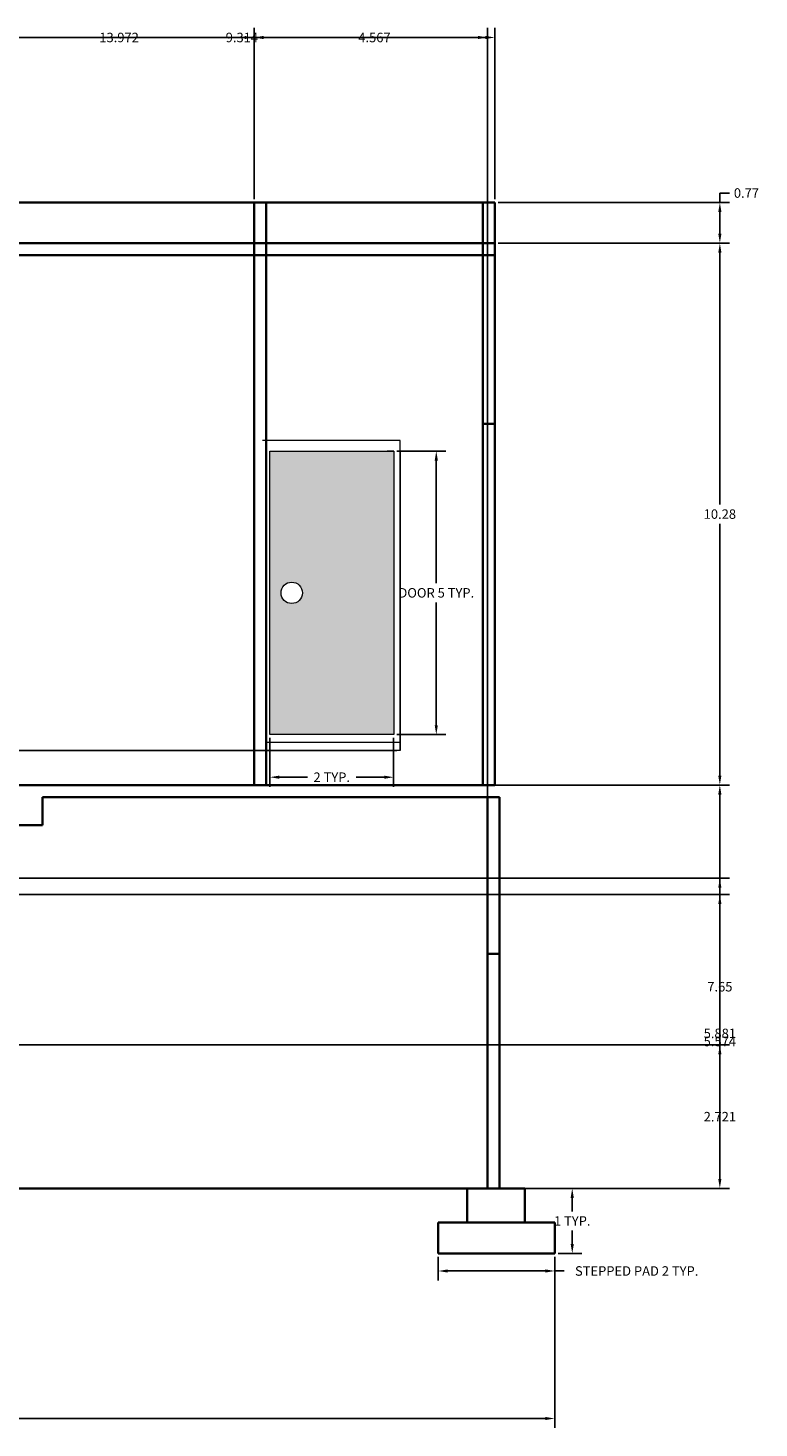
# Model space of a CAD drawing. Units: metres. Extents: x 1976.6 to 2045, y 823.7 to 850.3.
# Tile 3 of 3: x 2031.2 to 2045, y 823.7 to 850.3. Entities that reach past the tile are written whole.
import ezdxf

# ---------------------------------------------------------------- set-up
doc = ezdxf.new("R2010")
doc.units = ezdxf.units.M
for name, color, linetype, lineweight in [('A-ANNO-DIMS', 2, 'Continuous', 18), ('A-DOOR', 3, 'Continuous', 18), ('A-FLOR', 7, 'Continuous', 35), ('A-ROOF', 7, 'Continuous', 35), ('A-WALL', 7, 'Continuous', 35), ('A-WALL-PRPT', 7, 'Continuous', 35), ('S-BEAM', 1, 'Continuous', 35), ('S-FNDN', 1, 'Continuous', 35)]:
    doc.layers.add(name, color=color, linetype=linetype, lineweight=lineweight)
doc.styles.get("Standard").update_dxf_attribs({"font": 'arial.ttf'})
doc.dimstyles.get("Standard").update_dxf_attribs({"dimtxt": 0.18, "dimasz": 0.18, "dimexe": 0.18, "dimexo": 0.0625, "dimgap": 0.09, "dimtad": 0, "dimtih": 1, "dimtoh": 1, "dimdec": 4, "dimzin": 0, "dimdsep": 46, "dimtxsty": 'Standard', "dimcen": 0.09, "dimadec": 0, "dimazin": 0, "dimtfac": 1, "dimtdec": 4, "dimtofl": 0, "dimtmove": 0, "dimatfit": 3, "dimfxl": 1, "dimtolj": 1, "dimtzin": 0, "dimarcsym": 0})

# ---------------------------------------------------------------- blocks, each defined once
blk = doc.blocks.new('FNDN-STEPPED-PAD')
for p, q in [((0.547, 1.235), (0.547, 0.59)), ((1.641, 0.59), (1.641, 1.235)), ((0.547, 0.59), (0, 0.59)), ((0, 0.59), (0, 0)), ((0.547, 0.59), (1.641, 0.59)), ((2.209, 0.59), (1.641, 0.59)), ((2.209, 0), (2.209, 0.59)), ((0, 0), (2.209, 0))]:
    blk.add_line(p, q)
blk = doc.blocks.new('DOOR-SINGLE-LEAF')
h = blk.add_hatch(color=256)
h.dxf.hatch_style = 1
h.paths.add_polyline_path([(2.349, 5.38), (2.224, 5.38), (0, 5.38), (0, 0), (2.349, 0)])
h.paths.add_polyline_path([(0.213, 2.69, -1), (0.619, 2.69, -1)], flags=16)
for p, q in [((2.349, 5.38), (2.224, 5.38)), ((2.224, 5.38), (2.349, 5.38)), ((2.349, 5.38), (2.349, 0)), ((2.349, 0), (0, 0))]:
    blk.add_line(p, q)
blk.add_lwpolyline([(0, 0), (0, 5.38), (2.349, 5.38)])
blk.add_circle((0.416, 2.69), 0.203)
blk = doc.blocks.new('*D6')
at = {"layer": 'A-ANNO-DIMS', "color": 0, "lineweight": -2, "transparency": 16777216}
for p, q in [((2038.945, 826.987), (2038.945, 826.538)), ((2041.154, 826.987), (2041.154, 826.538)), ((2039.125, 826.718), (2040.974, 826.718)), ((2041.154, 826.718), (2041.334, 826.718))]:
    blk.add_line(p, q, dxfattribs=at)
at = {"layer": 'A-ANNO-DIMS', "color": 0, "transparency": 16777216}
for points in [[(2039.125, 826.748), (2039.125, 826.688), (2038.945, 826.718)], [(2040.974, 826.748), (2040.974, 826.688), (2041.154, 826.718)]]:
    blk.add_solid(points, dxfattribs=at)
at = {"layer": 'Defpoints', "color": 0, "transparency": 16777216}
for p in [(2038.945, 827.05), (2041.154, 827.05), (2041.154, 826.718)]:
    blk.add_point(p, dxfattribs=at)
at = {"layer": 'A-ANNO-DIMS', "color": 0, "transparency": 16777216, "insert": (2042.707, 826.718), "char_height": 0.18, "attachment_point": 5}
blk.add_mtext('\\A1;STEPPED PAD 2 TYP.', dxfattribs=at)
blk = doc.blocks.new('*D7')
at = {"layer": 'A-ANNO-DIMS', "color": 0, "lineweight": -2, "transparency": 16777216}
for p, q in [((2041.216, 828.285), (2041.665, 828.285)), ((2041.485, 828.105), (2041.485, 827.848)), ((2041.485, 827.23), (2041.485, 827.487)), ((2041.216, 827.05), (2041.665, 827.05))]:
    blk.add_line(p, q, dxfattribs=at)
at = {"layer": 'A-ANNO-DIMS', "color": 0, "transparency": 16777216}
for points in [[(2041.455, 828.105), (2041.515, 828.105), (2041.485, 828.285)], [(2041.455, 827.23), (2041.515, 827.23), (2041.485, 827.05)]]:
    blk.add_solid(points, dxfattribs=at)
at = {"layer": 'Defpoints', "color": 0, "transparency": 16777216}
for p in [(2041.154, 828.285), (2041.485, 828.285), (2041.154, 827.05)]:
    blk.add_point(p, dxfattribs=at)
at = {"layer": 'A-ANNO-DIMS', "color": 0, "transparency": 16777216, "insert": (2041.485, 827.667), "char_height": 0.18, "attachment_point": 5}
blk.add_mtext('\\A1;1 TYP.', dxfattribs=at)
blk = doc.blocks.new('*D12')
at = {"layer": 'A-ANNO-DIMS', "color": 0, "lineweight": -2, "transparency": 16777216}
for p, q in [((2038.162, 842.271), (2039.087, 842.271)), ((2038.907, 842.091), (2038.907, 839.764)), ((2038.907, 837.071), (2038.907, 839.398)), ((2038.162, 836.891), (2039.087, 836.891))]:
    blk.add_line(p, q, dxfattribs=at)
at = {"layer": 'A-ANNO-DIMS', "color": 0, "transparency": 16777216}
for points in [[(2038.877, 842.091), (2038.937, 842.091), (2038.907, 842.271)], [(2038.877, 837.071), (2038.937, 837.071), (2038.907, 836.891)]]:
    blk.add_solid(points, dxfattribs=at)
at = {"layer": 'Defpoints', "color": 0, "transparency": 16777216}
for p in [(2038.099, 842.271), (2038.907, 842.271), (2038.099, 836.891)]:
    blk.add_point(p, dxfattribs=at)
at = {"layer": 'A-ANNO-DIMS', "color": 0, "transparency": 16777216, "insert": (2038.907, 839.581), "char_height": 0.18, "attachment_point": 5}
blk.add_mtext('\\A1;DOOR 5 TYP.', dxfattribs=at)
blk = doc.blocks.new('*D13')
at = {"layer": 'A-ANNO-DIMS', "color": 0, "lineweight": -2, "transparency": 16777216}
for p, q in [((2035.75, 836.828), (2035.75, 835.904)), ((2038.099, 836.828), (2038.099, 835.904)), ((2035.93, 836.084), (2036.465, 836.084)), ((2037.919, 836.084), (2037.385, 836.084))]:
    blk.add_line(p, q, dxfattribs=at)
at = {"layer": 'A-ANNO-DIMS', "color": 0, "transparency": 16777216}
for points in [[(2035.93, 836.114), (2035.93, 836.054), (2035.75, 836.084)], [(2037.919, 836.114), (2037.919, 836.054), (2038.099, 836.084)]]:
    blk.add_solid(points, dxfattribs=at)
at = {"layer": 'Defpoints', "color": 0, "transparency": 16777216}
for p in [(2035.75, 836.891), (2038.099, 836.891), (2038.099, 836.084)]:
    blk.add_point(p, dxfattribs=at)
at = {"layer": 'A-ANNO-DIMS', "color": 0, "transparency": 16777216, "insert": (2036.925, 836.084), "char_height": 0.18, "attachment_point": 5}
blk.add_mtext('\\A1;2 TYP.', dxfattribs=at)
blk = doc.blocks.new('*D16')
at = {"layer": 'A-ANNO-DIMS', "color": 0, "lineweight": -2, "transparency": 16777216}
for p, q in [((1993.695, 826.987), (1993.695, 823.74)), ((2041.154, 826.987), (2041.154, 823.74)), ((1993.875, 823.92), (2017.027, 823.92)), ((2040.974, 823.92), (2017.822, 823.92))]:
    blk.add_line(p, q, dxfattribs=at)
at = {"layer": 'A-ANNO-DIMS', "color": 0, "transparency": 16777216}
for points in [[(1993.875, 823.95), (1993.875, 823.89), (1993.695, 823.92)], [(2040.974, 823.95), (2040.974, 823.89), (2041.154, 823.92)]]:
    blk.add_solid(points, dxfattribs=at)
at = {"layer": 'Defpoints', "color": 0, "transparency": 16777216}
for p in [(1993.695, 827.05), (2041.154, 827.05), (2041.154, 823.92)]:
    blk.add_point(p, dxfattribs=at)
at = {"layer": 'A-ANNO-DIMS', "color": 0, "transparency": 16777216, "insert": (2017.425, 823.92), "char_height": 0.18, "attachment_point": 5}
blk.add_mtext('\\A1;47.46', dxfattribs=at)
blk = doc.blocks.new('*D21')
at = {"layer": 'A-ANNO-DIMS', "color": 0, "lineweight": -2, "transparency": 16777216}
for p, q in [((2019.995, 847.047), (2019.995, 850.295)), ((2035.451, 847.047), (2035.451, 850.295)), ((2020.175, 850.115), (2027.268, 850.115)), ((2035.271, 850.115), (2028.178, 850.115))]:
    blk.add_line(p, q, dxfattribs=at)
at = {"layer": 'A-ANNO-DIMS', "color": 0, "transparency": 16777216}
for points in [[(2020.175, 850.145), (2020.175, 850.085), (2019.995, 850.115)], [(2035.271, 850.145), (2035.271, 850.085), (2035.451, 850.115)]]:
    blk.add_solid(points, dxfattribs=at)
at = {"layer": 'Defpoints', "color": 0, "transparency": 16777216}
for p in [(2035.451, 850.115), (2019.995, 846.985), (2035.451, 846.985)]:
    blk.add_point(p, dxfattribs=at)
at = {"layer": 'A-ANNO-DIMS', "color": 0, "transparency": 16777216, "insert": (2027.723, 850.115), "char_height": 0.18, "attachment_point": 5}
blk.add_mtext('\\A1;15.456', dxfattribs=at)
blk = doc.blocks.new('*D22')
at = {"layer": 'A-ANNO-DIMS', "color": 0, "lineweight": -2, "transparency": 16777216}
for p, q in [((2035.451, 847.047), (2035.451, 850.295)), ((2040.018, 847.047), (2040.018, 850.295)), ((2035.631, 850.115), (2037.337, 850.115)), ((2039.838, 850.115), (2038.132, 850.115))]:
    blk.add_line(p, q, dxfattribs=at)
at = {"layer": 'A-ANNO-DIMS', "color": 0, "transparency": 16777216}
for points in [[(2035.631, 850.145), (2035.631, 850.085), (2035.451, 850.115)], [(2039.838, 850.145), (2039.838, 850.085), (2040.018, 850.115)]]:
    blk.add_solid(points, dxfattribs=at)
at = {"layer": 'Defpoints', "color": 0, "transparency": 16777216}
for p in [(2040.018, 850.115), (2035.451, 846.985), (2040.018, 846.985)]:
    blk.add_point(p, dxfattribs=at)
at = {"layer": 'A-ANNO-DIMS', "color": 0, "transparency": 16777216, "insert": (2037.735, 850.115), "char_height": 0.18, "attachment_point": 5}
blk.add_mtext('\\A1;4.567', dxfattribs=at)
blk = doc.blocks.new('*D23')
at = {"layer": 'A-ANNO-DIMS', "color": 0, "lineweight": -2, "transparency": 16777216}
for p, q in [((2006.71, 835.935), (2044.464, 835.935)), ((2044.284, 835.755), (2044.284, 832.292)), ((2044.284, 828.465), (2044.284, 831.928)), ((2006.71, 828.285), (2044.464, 828.285))]:
    blk.add_line(p, q, dxfattribs=at)
at = {"layer": 'A-ANNO-DIMS', "color": 0, "transparency": 16777216}
for points in [[(2044.254, 835.755), (2044.314, 835.755), (2044.284, 835.935)], [(2044.254, 828.465), (2044.314, 828.465), (2044.284, 828.285)]]:
    blk.add_solid(points, dxfattribs=at)
at = {"layer": 'Defpoints', "color": 0, "transparency": 16777216}
for p in [(2006.648, 835.935), (2044.284, 835.935), (2006.648, 828.285)]:
    blk.add_point(p, dxfattribs=at)
at = {"layer": 'A-ANNO-DIMS', "color": 0, "transparency": 16777216, "insert": (2044.284, 832.11), "char_height": 0.18, "attachment_point": 5}
blk.add_mtext('\\A1;7.65', dxfattribs=at)
blk = doc.blocks.new('*D24')
at = {"layer": 'A-ANNO-DIMS', "color": 0, "lineweight": -2, "transparency": 16777216}
for p, q in [((2040.081, 846.215), (2044.464, 846.215)), ((2044.284, 846.035), (2044.284, 841.257)), ((2044.284, 836.115), (2044.284, 840.893)), ((2040.081, 835.935), (2044.464, 835.935))]:
    blk.add_line(p, q, dxfattribs=at)
at = {"layer": 'A-ANNO-DIMS', "color": 0, "transparency": 16777216}
for points in [[(2044.254, 846.035), (2044.314, 846.035), (2044.284, 846.215)], [(2044.254, 836.115), (2044.314, 836.115), (2044.284, 835.935)]]:
    blk.add_solid(points, dxfattribs=at)
at = {"layer": 'Defpoints', "color": 0, "transparency": 16777216}
for p in [(2040.018, 846.215), (2044.284, 846.215), (2040.018, 835.935)]:
    blk.add_point(p, dxfattribs=at)
at = {"layer": 'A-ANNO-DIMS', "color": 0, "transparency": 16777216, "insert": (2044.284, 841.075), "char_height": 0.18, "attachment_point": 5}
blk.add_mtext('\\A1;10.28', dxfattribs=at)
blk = doc.blocks.new('*D25')
at = {"layer": 'A-ANNO-DIMS', "color": 0, "lineweight": -2, "transparency": 16777216}
for p, q in [((2044.284, 846.985), (2044.284, 847.165)), ((2044.284, 847.165), (2044.464, 847.165)), ((2040.081, 846.985), (2044.464, 846.985)), ((2044.284, 846.395), (2044.284, 846.805)), ((2040.081, 846.215), (2044.464, 846.215))]:
    blk.add_line(p, q, dxfattribs=at)
at = {"layer": 'A-ANNO-DIMS', "color": 0, "transparency": 16777216}
for points in [[(2044.254, 846.805), (2044.314, 846.805), (2044.284, 846.985)], [(2044.254, 846.395), (2044.314, 846.395), (2044.284, 846.215)]]:
    blk.add_solid(points, dxfattribs=at)
at = {"layer": 'Defpoints', "color": 0, "transparency": 16777216}
for p in [(2040.018, 846.985), (2044.284, 846.985), (2040.018, 846.215)]:
    blk.add_point(p, dxfattribs=at)
at = {"layer": 'A-ANNO-DIMS', "color": 0, "transparency": 16777216, "insert": (2044.788, 847.165), "char_height": 0.18, "attachment_point": 5}
blk.add_mtext('\\A1;0.77', dxfattribs=at)
blk = doc.blocks.new('*D30')
at = {"layer": 'A-ANNO-DIMS', "color": 0, "lineweight": -2, "transparency": 16777216}
for p, q in [((2025.906, 828.347), (2025.906, 850.295)), ((2039.878, 828.347), (2039.878, 850.295)), ((2026.086, 850.115), (2032.437, 850.115)), ((2039.698, 850.115), (2033.346, 850.115))]:
    blk.add_line(p, q, dxfattribs=at)
at = {"layer": 'A-ANNO-DIMS', "color": 0, "transparency": 16777216}
for points in [[(2026.086, 850.145), (2026.086, 850.085), (2025.906, 850.115)], [(2039.698, 850.145), (2039.698, 850.085), (2039.878, 850.115)]]:
    blk.add_solid(points, dxfattribs=at)
at = {"layer": 'Defpoints', "color": 0, "transparency": 16777216}
for p in [(2039.878, 850.115), (2025.906, 828.285), (2039.878, 828.285)]:
    blk.add_point(p, dxfattribs=at)
at = {"layer": 'A-ANNO-DIMS', "color": 0, "transparency": 16777216, "insert": (2032.892, 850.115), "char_height": 0.18, "attachment_point": 5}
blk.add_mtext('\\A1;13.972', dxfattribs=at)
blk = doc.blocks.new('*D32')
at = {"layer": 'A-ANNO-DIMS', "color": 0, "lineweight": -2, "transparency": 16777216}
for p, q in [((1997.363, 831.006), (2044.464, 831.006)), ((2044.284, 830.826), (2044.284, 829.826)), ((2044.284, 828.465), (2044.284, 829.465)), ((1994.937, 828.285), (2044.464, 828.285))]:
    blk.add_line(p, q, dxfattribs=at)
at = {"layer": 'A-ANNO-DIMS', "color": 0, "transparency": 16777216}
for points in [[(2044.254, 830.826), (2044.314, 830.826), (2044.284, 831.006)], [(2044.254, 828.465), (2044.314, 828.465), (2044.284, 828.285)]]:
    blk.add_solid(points, dxfattribs=at)
at = {"layer": 'Defpoints', "color": 0, "transparency": 16777216}
for p in [(1997.3, 831.006), (1994.875, 828.285), (2044.284, 828.285)]:
    blk.add_point(p, dxfattribs=at)
at = {"layer": 'A-ANNO-DIMS', "color": 0, "transparency": 16777216, "insert": (2044.284, 829.645), "char_height": 0.18, "attachment_point": 5}
blk.add_mtext('\\A1;2.721', dxfattribs=at)
blk = doc.blocks.new('*D38')
at = {"layer": 'A-ANNO-DIMS', "color": 0, "lineweight": -2, "transparency": 16777216}
for p, q in [((2005.369, 834.166), (2044.464, 834.166)), ((2044.284, 833.986), (2044.284, 831.407)), ((2044.284, 828.465), (2044.284, 831.043)), ((2005.369, 828.285), (2044.464, 828.285))]:
    blk.add_line(p, q, dxfattribs=at)
at = {"layer": 'A-ANNO-DIMS', "color": 0, "transparency": 16777216}
for points in [[(2044.254, 833.986), (2044.314, 833.986), (2044.284, 834.166)], [(2044.254, 828.465), (2044.314, 828.465), (2044.284, 828.285)]]:
    blk.add_solid(points, dxfattribs=at)
at = {"layer": 'Defpoints', "color": 0, "transparency": 16777216}
for p in [(2005.307, 834.166), (2005.307, 828.285), (2044.284, 828.285)]:
    blk.add_point(p, dxfattribs=at)
at = {"layer": 'A-ANNO-DIMS', "color": 0, "transparency": 16777216, "insert": (2044.284, 831.225), "char_height": 0.18, "attachment_point": 5}
blk.add_mtext('\\A1;5.881', dxfattribs=at)
blk = doc.blocks.new('*D43')
at = {"layer": 'A-ANNO-DIMS', "color": 0, "lineweight": -2, "transparency": 16777216}
for p, q in [((2030.564, 832.99), (2030.564, 850.295)), ((2039.878, 832.797), (2039.878, 850.295)), ((2030.744, 850.115), (2034.827, 850.115)), ((2039.698, 850.115), (2035.614, 850.115))]:
    blk.add_line(p, q, dxfattribs=at)
at = {"layer": 'A-ANNO-DIMS', "color": 0, "transparency": 16777216}
for points in [[(2030.744, 850.145), (2030.744, 850.085), (2030.564, 850.115)], [(2039.698, 850.145), (2039.698, 850.085), (2039.878, 850.115)]]:
    blk.add_solid(points, dxfattribs=at)
at = {"layer": 'Defpoints', "color": 0, "transparency": 16777216}
for p in [(2039.878, 850.115), (2030.564, 832.927), (2039.878, 832.735)]:
    blk.add_point(p, dxfattribs=at)
at = {"layer": 'A-ANNO-DIMS', "color": 0, "transparency": 16777216, "insert": (2035.221, 850.115), "char_height": 0.18, "attachment_point": 5}
blk.add_mtext('\\A1;9.314', dxfattribs=at)
blk = doc.blocks.new('*D47')
at = {"layer": 'A-ANNO-DIMS', "color": 0, "lineweight": -2, "transparency": 16777216}
for p, q in [((2023.482, 833.859), (2044.464, 833.859)), ((2044.284, 833.679), (2044.284, 831.253)), ((2044.284, 828.465), (2044.284, 830.89)), ((2025.738, 828.285), (2044.464, 828.285))]:
    blk.add_line(p, q, dxfattribs=at)
at = {"layer": 'A-ANNO-DIMS', "color": 0, "transparency": 16777216}
for points in [[(2044.254, 833.679), (2044.314, 833.679), (2044.284, 833.859)], [(2044.254, 828.465), (2044.314, 828.465), (2044.284, 828.285)]]:
    blk.add_solid(points, dxfattribs=at)
at = {"layer": 'Defpoints', "color": 0, "transparency": 16777216}
for p in [(2023.419, 833.859), (2025.676, 828.285), (2044.284, 828.285)]:
    blk.add_point(p, dxfattribs=at)
at = {"layer": 'A-ANNO-DIMS', "color": 0, "transparency": 16777216, "insert": (2044.284, 831.072), "char_height": 0.18, "attachment_point": 5}
blk.add_mtext('\\A1;5.574', dxfattribs=at)
blk = doc.blocks.new('*D48')
at = {"layer": 'A-ANNO-DIMS', "color": 0, "lineweight": -2, "transparency": 16777216}
for p, q in [((2038.162, 836.589), (1986.237, 836.589)), ((1986.417, 836.409), (1986.417, 836.115)), ((2039.726, 835.935), (1986.237, 835.935)), ((1986.417, 835.755), (1986.237, 835.755)), ((1986.417, 835.935), (1986.417, 835.755))]:
    blk.add_line(p, q, dxfattribs=at)
at = {"layer": 'A-ANNO-DIMS', "color": 0, "transparency": 16777216}
for points in [[(1986.387, 836.409), (1986.447, 836.409), (1986.417, 836.589)], [(1986.387, 836.115), (1986.447, 836.115), (1986.417, 835.935)]]:
    blk.add_solid(points, dxfattribs=at)
at = {"layer": 'Defpoints', "color": 0, "transparency": 16777216}
for p in [(2038.224, 836.589), (1986.417, 835.935), (2039.788, 835.935)]:
    blk.add_point(p, dxfattribs=at)
at = {"layer": 'A-ANNO-DIMS', "color": 0, "transparency": 16777216, "insert": (1985.913, 835.755), "char_height": 0.18, "attachment_point": 5}
blk.add_mtext('\\A1;0.65', dxfattribs=at)

msp = doc.modelspace()

# ---------------------------------------------------------------- linework, layer by layer
at = {"layer": 'A-DOOR'}
for p, q in [((2038.2243, 842.4695), (2035.61, 842.4695)), ((2038.2243, 836.5887), (2038.2243, 842.4695)), ((2035.6811, 836.751), (2038.2243, 836.751)), ((2035.7503, 836.5887), (2035.6811, 836.5887))]:
    msp.add_line(p, q, dxfattribs=at)
msp.add_lwpolyline([(2038.2243, 842.2713), (2038.2243, 836.5887), (2035.7503, 836.5887)], dxfattribs=at)
at = {"layer": 'A-FLOR'}
for p, q in [((2019.9947, 835.9348), (2040.0184, 835.9348)), ((2040.1075, 835.7048), (2031.4404, 835.7048)), ((2031.4404, 835.7048), (2040.1075, 835.7048)), ((2040.5852, 828.2848), (1993.0497, 828.2848)), ((2040.5852, 828.2848), (1994.6446, 828.2848))]:
    msp.add_line(p, q, dxfattribs=at)
at = {"layer": 'A-ROOF'}
for p, q in [((2040.0184, 846.2148), (1993.6952, 846.2148)), ((2006.6479, 845.9848), (2040.0184, 845.9848)), ((2040.0184, 845.9848), (2006.6479, 845.9848))]:
    msp.add_line(p, q, dxfattribs=at)
at = {"layer": 'A-WALL'}
for p, q in [((2035.4511, 846.9848), (2035.4511, 835.9348)), ((2035.6811, 846.9848), (2035.6811, 835.9348)), ((2039.7884, 846.9848), (2039.7884, 835.9348)), ((2040.0184, 846.9848), (2040.0184, 835.9348)), ((2039.7884, 842.7848), (2040.0184, 842.7848)), ((2039.8775, 834.7023), (2039.8775, 835.7048)), ((2039.8775, 835.7048), (2040.1075, 835.7048)), ((2040.1075, 834.6169), (2040.1075, 835.7048)), ((2039.8775, 834.7023), (2039.8775, 828.2848)), ((2040.1075, 834.7023), (2040.1075, 828.2848)), ((2040.1075, 834.7023), (2040.1075, 834.6169)), ((2039.8775, 832.7348), (2040.1075, 832.7348))]:
    msp.add_line(p, q, dxfattribs=at)
at = {"layer": 'A-WALL-PRPT'}
msp.add_line((2040.0184, 846.9848), (1994.6446, 846.9848), dxfattribs=at)
at = {"layer": 'S-BEAM'}
for p, q in [((2031.4404, 835.1735), (2031.4404, 835.7048)), ((2030.8908, 835.1735), (2031.4404, 835.1735))]:
    msp.add_line(p, q, dxfattribs=at)

# ---------------------------------------------------------------- block references
at = {"layer": 'A-DOOR'}
msp.add_blockref('DOOR-SINGLE-LEAF', (2035.7506, 836.8909), dxfattribs=at)
at = {"layer": 'S-FNDN'}
msp.add_blockref('FNDN-STEPPED-PAD', (2038.9447, 827.05), dxfattribs=at)

# ---------------------------------------------------------------- dimensions: what is measured, and where the dimension line sits
at = {"layer": 'A-ANNO-DIMS'}
for base, p1, p2, override, picture, middle in [((2035.4511, 850.1148), (2019.9947, 846.9848), (2035.4511, 846.9848), {"dimdec": 3, "dimlfac": 1, "dimrnd": 0, "dimzin": 0, "dimdsep": 46, "dimlunit": 2}, '*D21', (2027.7229, 850.1148)), ((2039.8775, 850.1148), (2025.9056, 828.2848), (2039.8775, 828.2848), {"dimdec": 3, "dimlfac": 1, "dimrnd": 0, "dimzin": 0, "dimdsep": 46, "dimlunit": 2}, '*D30', (2032.8915, 850.1148)), ((2039.8775, 850.1148), (2030.5639, 832.9273), (2039.8775, 832.7348), {"dimdec": 3, "dimlfac": 1, "dimrnd": 0, "dimzin": 0, "dimdsep": 46, "dimlunit": 2}, '*D43', (2035.2207, 850.1148)), ((2040.0184, 850.1148), (2035.4511, 846.9848), (2040.0184, 846.9848), {"dimdec": 3, "dimlfac": 1, "dimrnd": 0, "dimzin": 0, "dimdsep": 46, "dimlunit": 2}, '*D22', (2037.7347, 850.1148)), ((2041.1538, 823.9197), (1993.6952, 827.0497), (2041.1538, 827.0497), {"dimdec": 2, "dimlfac": 1, "dimrnd": 0, "dimzin": 0, "dimdsep": 46, "dimlunit": 2}, '*D16', (2017.4245, 823.9197))]:
    dim = msp.add_linear_dim(base=base, p1=p1, p2=p2, dimstyle='Standard', override=override, dxfattribs=at)
    dim.commit()
    dim.dimension.update_dxf_attribs({"geometry": picture, "text_midpoint": middle})
for base, p1, p2, override, picture, middle in [((2044.2838, 846.9848), (2040.0184, 846.2148), (2040.0184, 846.9848), {"dimdec": 2, "dimlfac": 1, "dimrnd": 0, "dimzin": 0, "dimdsep": 46, "dimlunit": 2}, '*D25', (2044.7876, 847.1648)), ((2044.2838, 846.2148), (2040.0184, 835.9348), (2040.0184, 846.2148), {"dimdec": 2, "dimlfac": 1, "dimrnd": 0, "dimzin": 0, "dimdsep": 46, "dimlunit": 2}, '*D24', (2044.2838, 841.0748)), ((1986.4174, 835.9348), (2038.2243, 836.5887), (2039.7884, 835.9348), {"dimdec": 2, "dimlfac": 1, "dimrnd": 0, "dimzin": 0, "dimdsep": 46, "dimlunit": 2}, '*D48', (1985.913, 835.7548)), ((2044.2838, 835.9348), (2006.6479, 828.2848), (2006.6479, 835.9348), {"dimdec": 2, "dimlfac": 1, "dimrnd": 0, "dimzin": 0, "dimdsep": 46, "dimlunit": 2}, '*D23', (2044.2838, 832.1098)), ((2044.2838, 828.2848), (2005.3067, 834.1656), (2005.3067, 828.2848), {"dimdec": 3, "dimlfac": 1, "dimrnd": 0, "dimzin": 0, "dimdsep": 46, "dimlunit": 2}, '*D38', (2044.2838, 831.2252)), ((2044.2838, 828.2848), (2023.4194, 833.8587), (2025.6756, 828.2848), {"dimdec": 3, "dimlfac": 1, "dimrnd": 0, "dimzin": 0, "dimdsep": 46, "dimlunit": 2}, '*D47', (2044.2838, 831.0718)), ((2044.2838, 828.2848), (1997.3001, 831.0057), (1994.8746, 828.2848), {"dimdec": 3, "dimlfac": 1, "dimrnd": 0, "dimzin": 0, "dimdsep": 46, "dimlunit": 2}, '*D32', (2044.2838, 829.6453))]:
    dim = msp.add_linear_dim(base=base, p1=p1, p2=p2, angle=90, dimstyle='Standard', override=override, dxfattribs=at)
    dim.commit()
    dim.dimension.update_dxf_attribs({"geometry": picture, "text_midpoint": middle})
for base, p1, p2, text, picture, middle in [((2038.9065, 842.2713), (2038.0994, 836.8906), (2038.0994, 842.2713), 'DOOR <> TYP.', '*D12', (2038.9065, 839.581)), ((2041.4852, 828.2848), (2041.1538, 827.0497), (2041.1538, 828.2848), '<> TYP.', '*D7', (2041.4852, 827.6673))]:
    dim = msp.add_linear_dim(base=base, p1=p1, p2=p2, angle=90, text=text, dimstyle='Standard', override={"dimdec": 0, "dimlfac": 1, "dimrnd": 0, "dimzin": 0, "dimdsep": 46, "dimlunit": 2}, dxfattribs=at)
    dim.commit()
    dim.dimension.update_dxf_attribs({"geometry": picture, "text_midpoint": middle})
for base, p1, p2, text, picture, middle in [((2038.0994, 836.0835), (2035.7503, 836.8906), (2038.0994, 836.8906), '<> TYP.', '*D13', (2036.9248, 836.0835)), ((2041.1538, 826.7184), (2038.9449, 827.0497), (2041.1538, 827.0497), 'STEPPED PAD <> TYP.', '*D6', (2042.7068, 826.7184))]:
    dim = msp.add_linear_dim(base=base, p1=p1, p2=p2, text=text, dimstyle='Standard', override={"dimdec": 0, "dimlfac": 1, "dimrnd": 0, "dimzin": 0, "dimdsep": 46, "dimlunit": 2}, dxfattribs=at)
    dim.commit()
    dim.dimension.update_dxf_attribs({"geometry": picture, "text_midpoint": middle})

doc.saveas('drawing.dxf')
